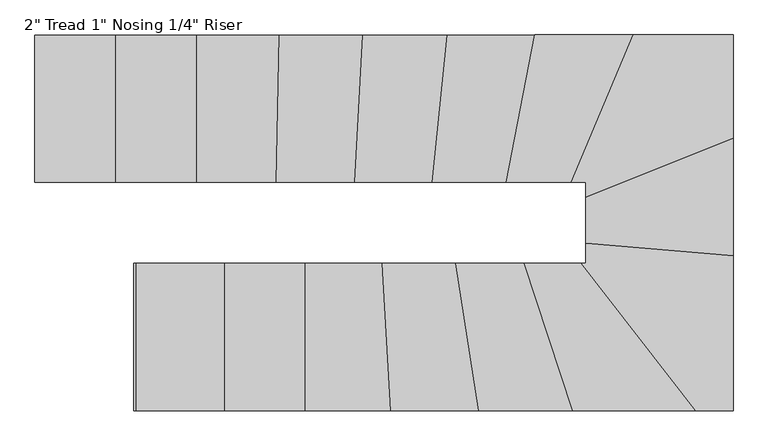
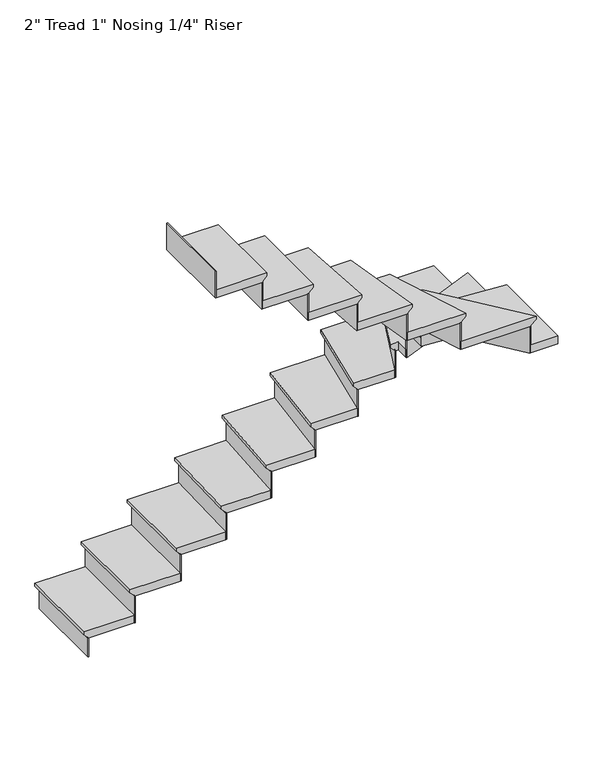
"""IFC4 building model written with IfcOpenShell, lengths in millimetres: stair flight geometry."""

from ifc_helpers import new_model, si_unit, origin, place, context, project, spatial, faceted_brep, source, transform, mapped, element, save


def stair_flight_0d7771ed(model_context):
    return source(origin(), model_context, "Body", "Brep", [
        faceted_brep([(838.4202681, 2693.877558, 9920.8166667), (838.4202681, 2693.877558, 9939.8666667), (838.4202681, 3202.4524989, 9939.8666667), (838.4202681, 3202.4524989, 9920.8166667), (863.8202681, 2693.877558, 9895.4166667), (863.8202681, 3202.4524989, 9895.4166667), (1143.2202681, 2693.877558, 9939.8666667), (1143.2202681, 3202.4524989, 9939.8666667), (863.8202681, 3202.4524989, 9889.0666667), (1143.2202681, 3202.4524989, 9889.0666667), (1143.2202681, 2693.877558, 9889.0666667), (863.8202681, 2693.877558, 9889.0666667)], [[[0, 1, 2, 3]], [[4, 0, 3, 5]], [[2, 1, 6, 7]], [[8, 9, 10, 11]], [[2, 7, 9, 8, 5, 3]], [[8, 11, 4, 5]], [[6, 1, 0, 4, 11, 10]], [[7, 6, 10, 9]]]),
        faceted_brep([(863.8202681, 2693.877558, 9889.0666667), (863.8202681, 2693.877558, 9770.5333333), (870.1702681, 2693.877558, 9770.5333333), (870.1702681, 2693.877558, 9889.0666667), (863.8202681, 3202.4524989, 9889.0666667), (870.1702681, 3202.4524989, 9889.0666667), (870.1702681, 3202.4524989, 9770.5333333), (863.8202681, 3202.4524989, 9770.5333333)], [[[0, 1, 2, 3]], [[4, 5, 6, 7]], [[1, 0, 4, 7]], [[2, 1, 7, 6]], [[3, 2, 6, 5]], [[0, 3, 5, 4]]]),
        faceted_brep([(1143.2202681, 2693.877558, 10058.4), (1143.2202681, 2693.877558, 9889.0666667), (1149.5702681, 2693.877558, 9889.0666667), (1149.5702681, 2693.877558, 10058.4), (1143.2202681, 3202.4524989, 10058.4), (1149.5702681, 3202.4524989, 10058.4), (1149.5702681, 3202.4524989, 9889.0666667), (1143.2202681, 3202.4524989, 9889.0666667)], [[[0, 1, 2, 3]], [[4, 5, 6, 7]], [[1, 0, 4, 7]], [[2, 1, 7, 6]], [[3, 2, 6, 5]], [[0, 3, 5, 4]]]),
        faceted_brep([(1117.8202681, 3202.4524989, 10109.2), (1117.8202681, 2693.877558, 10109.2), (1422.6202681, 2693.877558, 10109.2), (1422.6202681, 3202.4524989, 10109.2), (1143.2202681, 3202.4524989, 10058.4), (1422.6202681, 3202.4524989, 10058.4), (1422.6202681, 2693.877558, 10058.4), (1143.2202681, 2693.877558, 10058.4), (1143.2202681, 3202.4524989, 10064.75), (1117.8202681, 3202.4524989, 10090.15), (1143.2202681, 2693.877558, 10064.75), (1117.8202681, 2693.877558, 10090.15)], [[[0, 1, 2, 3]], [[4, 5, 6, 7]], [[0, 3, 5, 4, 8, 9]], [[4, 7, 10, 8]], [[2, 1, 11, 10, 7, 6]], [[3, 2, 6, 5]], [[11, 1, 0, 9]], [[10, 11, 9, 8]]]),
        faceted_brep([(1422.6202681, 2693.877558, 10227.7333333), (1422.6202681, 2693.877558, 10058.4), (1428.9702681, 2693.877558, 10058.4), (1428.9702681, 2693.877558, 10227.7333333), (1422.6202681, 3202.4524989, 10227.7333333), (1428.9702681, 3202.4524989, 10227.7333333), (1428.9702681, 3202.4524989, 10058.4), (1422.6202681, 3202.4524989, 10058.4)], [[[0, 1, 2, 3]], [[4, 5, 6, 7]], [[1, 0, 4, 7]], [[2, 1, 7, 6]], [[3, 2, 6, 5]], [[0, 3, 5, 4]]]),
        faceted_brep([(1397.2202681, 3202.4524989, 10278.5333333), (1397.2202681, 2693.877558, 10278.5333333), (1696.6553711, 2693.877558, 10278.5333333), (1707.3964935, 3202.4524989, 10278.5333333), (1422.6202681, 3202.4524989, 10227.7333333), (1707.3964935, 3202.4524989, 10227.7333333), (1696.6553711, 2693.877558, 10227.7333333), (1422.6202681, 2693.877558, 10227.7333333), (1422.6202681, 3202.4524989, 10234.0833333), (1397.2202681, 3202.4524989, 10259.4833333), (1422.6202681, 2693.877558, 10234.0833333), (1397.2202681, 2693.877558, 10259.4833333)], [[[0, 1, 2, 3]], [[4, 5, 6, 7]], [[0, 3, 5, 4, 8, 9]], [[4, 7, 10, 8]], [[2, 1, 11, 10, 7, 6]], [[3, 2, 6, 5]], [[11, 1, 0, 9]], [[10, 11, 9, 8]]]),
        faceted_brep([(1696.6553711, 2693.877558, 10397.0666667), (1696.6553711, 2693.877558, 10227.7333333), (1703.0067872, 2693.877558, 10227.7333333), (1703.0067872, 2693.877558, 10397.0666667), (1707.3964935, 3202.4524989, 10397.0666667), (1713.7479096, 3202.4524989, 10397.0666667), (1713.7479096, 3202.4524989, 10227.7333333), (1707.3964935, 3202.4524989, 10227.7333333)], [[[0, 1, 2, 3]], [[4, 5, 6, 7]], [[1, 0, 4, 7]], [[2, 1, 7, 6]], [[3, 2, 6, 5]], [[0, 3, 5, 4]]]),
        faceted_brep([(1681.9908293, 3202.4524989, 10447.8666667), (1671.2497068, 2693.877558, 10447.8666667), (1968.2389719, 2693.877558, 10447.8666667), (1994.6701229, 3202.4524989, 10447.8666667), (1707.3964935, 3202.4524989, 10397.0666667), (1994.6701229, 3202.4524989, 10397.0666667), (1968.2389719, 2693.877558, 10397.0666667), (1696.6553711, 2693.877558, 10397.0666667), (1707.3964935, 3202.4524989, 10403.4166667), (1681.9908293, 3202.4524989, 10428.8166667), (1696.6553711, 2693.877558, 10403.4166667), (1671.2497068, 2693.877558, 10428.8166667)], [[[0, 1, 2, 3]], [[4, 5, 6, 7]], [[0, 3, 5, 4, 8, 9]], [[4, 7, 10, 8]], [[2, 1, 11, 10, 7, 6]], [[3, 2, 6, 5]], [[11, 1, 0, 9]], [[10, 11, 9, 8]]]),
        faceted_brep([(1968.2389719, 2693.877558, 10566.4), (1968.2389719, 2693.877558, 10397.0666667), (1974.5975418, 2693.877558, 10397.0666667), (1974.5975418, 2693.877558, 10566.4), (1994.6701229, 3202.4524989, 10566.4), (2001.0286928, 3202.4524989, 10566.4), (2001.0286928, 3202.4524989, 10397.0666667), (1994.6701229, 3202.4524989, 10397.0666667)], [[[0, 1, 2, 3]], [[4, 5, 6, 7]], [[1, 0, 4, 7]], [[2, 1, 7, 6]], [[3, 2, 6, 5]], [[0, 3, 5, 4]]]),
        faceted_brep([(1969.2358436, 3202.4524989, 10617.2), (1942.8046925, 2693.877558, 10617.2), (2235.1931673, 2693.877558, 10617.2), (2286.7073051, 3202.4524989, 10617.2), (1994.6701229, 3202.4524989, 10566.4), (2286.7073051, 3202.4524989, 10566.4), (2235.1931673, 2693.877558, 10566.4), (1968.2389719, 2693.877558, 10566.4), (1994.6701229, 3202.4524989, 10572.75), (1969.2358436, 3202.4524989, 10598.15), (1968.2389719, 2693.877558, 10572.75), (1942.8046925, 2693.877558, 10598.15)], [[[0, 1, 2, 3]], [[4, 5, 6, 7]], [[0, 3, 5, 4, 8, 9]], [[4, 7, 10, 8]], [[2, 1, 11, 10, 7, 6]], [[3, 2, 6, 5]], [[11, 1, 0, 9]], [[10, 11, 9, 8]]]),
        faceted_brep([(2235.1931673, 2693.877558, 10735.7333333), (2235.1931673, 2693.877558, 10566.4), (2241.5756594, 2693.877558, 10566.4), (2241.5756594, 2693.877558, 10735.7333333), (2286.7073051, 3202.4524989, 10735.7333333), (2293.0897971, 3202.4524989, 10735.7333333), (2293.0897971, 3202.4524989, 10566.4), (2286.7073051, 3202.4524989, 10566.4)], [[[0, 1, 2, 3]], [[4, 5, 6, 7]], [[1, 0, 4, 7]], [[2, 1, 7, 6]], [[3, 2, 6, 5]], [[0, 3, 5, 4]]]),
        faceted_brep([(2261.1773369, 3202.4524989, 10786.5333333), (2209.6631992, 2693.877558, 10786.5333333), (2491.6737127, 2693.877558, 10786.5333333), (2589.7018996, 3202.4524989, 10786.5333333), (2286.7073051, 3202.4524989, 10735.7333333), (2589.7018996, 3202.4524989, 10735.7333333), (2491.6737127, 2693.877558, 10735.7333333), (2235.1931673, 2693.877558, 10735.7333333), (2286.7073051, 3202.4524989, 10742.0833333), (2261.1773369, 3202.4524989, 10767.4833333), (2235.1931673, 2693.877558, 10742.0833333), (2209.6631992, 2693.877558, 10767.4833333)], [[[0, 1, 2, 3]], [[4, 5, 6, 7]], [[0, 3, 5, 4, 8, 9]], [[4, 7, 10, 8]], [[2, 1, 11, 10, 7, 6]], [[3, 2, 6, 5]], [[11, 1, 0, 9]], [[10, 11, 9, 8]]]),
        faceted_brep([(2491.6737127, 2693.877558, 10905.0666667), (2491.6737127, 2693.877558, 10735.7333333), (2498.1405972, 2693.877558, 10735.7333333), (2498.1405972, 2693.877558, 10905.0666667), (2589.7018996, 3202.4524989, 10905.0666667), (2596.1687841, 3202.4524989, 10905.0666667), (2596.1687841, 3202.4524989, 10735.7333333), (2589.7018996, 3202.4524989, 10735.7333333)], [[[0, 1, 2, 3]], [[4, 5, 6, 7]], [[1, 0, 4, 7]], [[2, 1, 7, 6]], [[3, 2, 6, 5]], [[0, 3, 5, 4]]]),
        faceted_brep([(2563.8343615, 3202.4524989, 10955.8666667), (2465.8061746, 2693.877558, 10955.8666667), (2717.082711, 2693.877558, 10955.8666667), (2931.3822032, 3202.4524989, 10955.8666667), (2589.7018996, 3202.4524989, 10905.0666667), (2931.3822032, 3202.4524989, 10905.0666667), (2717.082711, 2693.877558, 10905.0666667), (2491.6737127, 2693.877558, 10905.0666667), (2589.7018996, 3202.4524989, 10911.4166667), (2563.8343615, 3202.4524989, 10936.8166667), (2491.6737127, 2693.877558, 10911.4166667), (2465.8061746, 2693.877558, 10936.8166667)], [[[0, 1, 2, 3]], [[4, 5, 6, 7]], [[0, 3, 5, 4, 8, 9]], [[4, 7, 10, 8]], [[2, 1, 11, 10, 7, 6]], [[3, 2, 6, 5]], [[11, 1, 0, 9]], [[10, 11, 9, 8]]]),
        faceted_brep([(2717.082711, 2693.877558, 11074.4), (2717.082711, 2693.877558, 10905.0666667), (2723.973426, 2693.877558, 10905.0666667), (2723.973426, 2693.877558, 11074.4), (2931.3822032, 3202.4524989, 11074.4), (2938.2729181, 3202.4524989, 11074.4), (2938.2729181, 3202.4524989, 10905.0666667), (2931.3822032, 3202.4524989, 10905.0666667)], [[[0, 1, 2, 3]], [[4, 5, 6, 7]], [[1, 0, 4, 7]], [[2, 1, 7, 6]], [[3, 2, 6, 5]], [[0, 3, 5, 4]]]),
        faceted_brep([(3247.982332, 2818.4435318, 11125.2), (3247.982332, 3202.4524989, 11125.2), (2903.8193433, 3202.4524989, 11125.2), (2689.5198512, 2693.877558, 11125.2), (2739.4073911, 2693.877558, 11125.2), (2739.4073911, 2614.5975609, 11125.2), (3247.982332, 3202.4524989, 11074.4), (3247.982332, 2818.4435318, 11074.4), (2739.4073911, 2614.5975609, 11074.4), (2739.4073911, 2693.877558, 11074.4), (2717.082711, 2693.877558, 11074.4), (2931.3822032, 3202.4524989, 11074.4), (2717.082711, 2693.877558, 11080.75), (2931.3822032, 3202.4524989, 11080.75), (2689.5198512, 2693.877558, 11106.15), (2903.8193433, 3202.4524989, 11106.15)], [[[0, 1, 2, 3, 4, 5]], [[6, 7, 8, 9, 10, 11]], [[1, 0, 7, 6]], [[11, 10, 12, 13]], [[5, 4, 9, 8]], [[0, 5, 8, 7]], [[14, 3, 2, 15]], [[12, 14, 15, 13]], [[4, 3, 14, 12, 10, 9]], [[2, 1, 6, 11, 13, 15]]]),
        faceted_brep([(2739.4073911, 2614.5975609, 11243.7333333), (2739.4073911, 2614.5975609, 11074.4), (2739.4073911, 2607.7564709, 11074.4), (2739.4073911, 2607.7564709, 11243.7333333), (3247.982332, 2818.4435318, 11243.7333333), (3247.982332, 2811.6024418, 11243.7333333), (3247.982332, 2811.6024418, 11074.4), (3247.982332, 2818.4435318, 11074.4)], [[[0, 1, 2, 3]], [[4, 5, 6, 7]], [[1, 0, 4, 7]], [[2, 1, 7, 6]], [[3, 2, 6, 5]], [[0, 3, 5, 4]]]),
        faceted_brep([(3247.982332, 2845.807892, 11294.5333333), (2739.4073911, 2641.9619211, 11294.5333333), (2739.4073911, 2458.7583414, 11294.5333333), (3247.982332, 2415.6151582, 11294.5333333), (3247.982332, 2818.4435318, 11243.7333333), (3247.982332, 2415.6151582, 11243.7333333), (2739.4073911, 2458.7583414, 11243.7333333), (2739.4073911, 2614.5975609, 11243.7333333), (3247.982332, 2818.4435318, 11250.0833333), (3247.982332, 2845.807892, 11275.4833333), (2739.4073911, 2614.5975609, 11250.0833333), (2739.4073911, 2641.9619211, 11275.4833333)], [[[0, 1, 2, 3]], [[4, 5, 6, 7]], [[0, 3, 5, 4, 8, 9]], [[4, 7, 10, 8]], [[2, 1, 11, 10, 7, 6]], [[3, 2, 6, 5]], [[11, 1, 0, 9]], [[10, 11, 9, 8]]]),
        faceted_brep([(2739.4073911, 2458.7583414, 11413.0666667), (2739.4073911, 2458.7583414, 11243.7333333), (2739.4073911, 2452.3855338, 11243.7333333), (2739.4073911, 2452.3855338, 11413.0666667), (3247.982332, 2415.6151582, 11413.0666667), (3247.982332, 2409.2423506, 11413.0666667), (3247.982332, 2409.2423506, 11243.7333333), (3247.982332, 2415.6151582, 11243.7333333)], [[[0, 1, 2, 3]], [[4, 5, 6, 7]], [[1, 0, 4, 7]], [[2, 1, 7, 6]], [[3, 2, 6, 5]], [[0, 3, 5, 4]]]),
        faceted_brep([(3085.5772675, 1905.9026171, 11463.8666667), (3247.982332, 1905.9026171, 11463.8666667), (3247.982332, 2441.1063885, 11463.8666667), (2739.4073911, 2484.2495716, 11463.8666667), (2739.4073911, 2414.477558, 11463.8666667), (2689.4386829, 2414.477558, 11463.8666667), (3247.982332, 1905.9026171, 11413.0666667), (3085.5772675, 1905.9026171, 11413.0666667), (2689.4386829, 2414.477558, 11413.0666667), (2739.4073911, 2414.477558, 11413.0666667), (2739.4073911, 2458.7583414, 11413.0666667), (3247.982332, 2415.6151582, 11413.0666667), (2739.4073911, 2458.7583414, 11419.4166667), (3247.982332, 2415.6151582, 11419.4166667), (2739.4073911, 2484.2495716, 11444.8166667), (3247.982332, 2441.1063885, 11444.8166667)], [[[0, 1, 2, 3, 4, 5]], [[6, 7, 8, 9, 10, 11]], [[1, 0, 7, 6]], [[11, 10, 12, 13]], [[4, 3, 14, 12, 10, 9]], [[5, 4, 9, 8]], [[0, 5, 8, 7]], [[14, 3, 2, 15]], [[12, 14, 15, 13]], [[2, 1, 6, 11, 13, 15]]]),
        faceted_brep([(2689.4386829, 2414.477558, 11582.4), (2689.4386829, 2414.477558, 11413.0666667), (2681.3896615, 2414.477558, 11413.0666667), (2681.3896615, 2414.477558, 11582.4), (3085.5772675, 1905.9026171, 11582.4), (3077.5282461, 1905.9026171, 11582.4), (3077.5282461, 1905.9026171, 11413.0666667), (3085.5772675, 1905.9026171, 11413.0666667)], [[[0, 1, 2, 3]], [[4, 5, 6, 7]], [[1, 0, 4, 7]], [[2, 1, 7, 6]], [[3, 2, 6, 5]], [[0, 3, 5, 4]]]),
        faceted_brep([(3117.7733531, 1905.9026171, 11633.2), (2721.6347685, 2414.477558, 11633.2), (2498.169104, 2414.477558, 11633.2), (2665.6971357, 1905.9026171, 11633.2), (3085.5772675, 1905.9026171, 11582.4), (2665.6971357, 1905.9026171, 11582.4), (2498.169104, 2414.477558, 11582.4), (2689.4386829, 2414.477558, 11582.4), (3085.5772675, 1905.9026171, 11588.75), (3117.7733531, 1905.9026171, 11614.15), (2689.4386829, 2414.477558, 11588.75), (2721.6347685, 2414.477558, 11614.15)], [[[0, 1, 2, 3]], [[4, 5, 6, 7]], [[0, 3, 5, 4, 8, 9]], [[4, 7, 10, 8]], [[2, 1, 11, 10, 7, 6]], [[3, 2, 6, 5]], [[11, 1, 0, 9]], [[10, 11, 9, 8]]]),
        faceted_brep([(2498.169104, 2414.477558, 11751.7333333), (2498.169104, 2414.477558, 11582.4), (2491.4834592, 2414.477558, 11582.4), (2491.4834592, 2414.477558, 11751.7333333), (2665.6971357, 1905.9026171, 11751.7333333), (2659.0114908, 1905.9026171, 11751.7333333), (2659.0114908, 1905.9026171, 11582.4), (2665.6971357, 1905.9026171, 11582.4)], [[[0, 1, 2, 3]], [[4, 5, 6, 7]], [[1, 0, 4, 7]], [[2, 1, 7, 6]], [[3, 2, 6, 5]], [[0, 3, 5, 4]]]),
        faceted_brep([(2692.4397151, 1905.9026171, 11802.5333333), (2524.9116834, 2414.477558, 11802.5333333), (2264.2527614, 2414.477558, 11802.5333333), (2342.8948816, 1905.9026171, 11802.5333333), (2665.6971357, 1905.9026171, 11751.7333333), (2342.8948816, 1905.9026171, 11751.7333333), (2264.2527614, 2414.477558, 11751.7333333), (2498.169104, 2414.477558, 11751.7333333), (2665.6971357, 1905.9026171, 11758.0833333), (2692.4397151, 1905.9026171, 11783.4833333), (2498.169104, 2414.477558, 11758.0833333), (2524.9116834, 2414.477558, 11783.4833333)], [[[0, 1, 2, 3]], [[4, 5, 6, 7]], [[0, 3, 5, 4, 8, 9]], [[4, 7, 10, 8]], [[2, 1, 11, 10, 7, 6]], [[3, 2, 6, 5]], [[11, 1, 0, 9]], [[10, 11, 9, 8]]]),
        faceted_brep([(2264.2527614, 2414.477558, 11921.0666667), (2264.2527614, 2414.477558, 11751.7333333), (2257.827292, 2414.477558, 11751.7333333), (2257.827292, 2414.477558, 11921.0666667), (2342.8948816, 1905.9026171, 11921.0666667), (2336.4694122, 1905.9026171, 11921.0666667), (2336.4694122, 1905.9026171, 11751.7333333), (2342.8948816, 1905.9026171, 11751.7333333)], [[[0, 1, 2, 3]], [[4, 5, 6, 7]], [[1, 0, 4, 7]], [[2, 1, 7, 6]], [[3, 2, 6, 5]], [[0, 3, 5, 4]]]),
        faceted_brep([(2368.5967594, 1905.9026171, 11971.8666667), (2289.9546392, 2414.477558, 11971.8666667), (2009.2587296, 2414.477558, 11971.8666667), (2039.6023306, 1905.9026171, 11971.8666667), (2342.8948816, 1905.9026171, 11921.0666667), (2039.6023306, 1905.9026171, 11921.0666667), (2009.2587296, 2414.477558, 11921.0666667), (2264.2527614, 2414.477558, 11921.0666667), (2342.8948816, 1905.9026171, 11927.4166667), (2368.5967594, 1905.9026171, 11952.8166667), (2264.2527614, 2414.477558, 11927.4166667), (2289.9546392, 2414.477558, 11952.8166667)], [[[0, 1, 2, 3]], [[4, 5, 6, 7]], [[0, 3, 5, 4, 8, 9]], [[4, 7, 10, 8]], [[2, 1, 11, 10, 7, 6]], [[3, 2, 6, 5]], [[11, 1, 0, 9]], [[10, 11, 9, 8]]]),
        faceted_brep([(2009.2587296, 2414.477558, 12090.4), (2009.2587296, 2414.477558, 11921.0666667), (2002.8974373, 2414.477558, 11921.0666667), (2002.8974373, 2414.477558, 12090.4), (2039.6023306, 1905.9026171, 12090.4), (2033.2410383, 1905.9026171, 12090.4), (2033.2410383, 1905.9026171, 11921.0666667), (2039.6023306, 1905.9026171, 11921.0666667)], [[[0, 1, 2, 3]], [[4, 5, 6, 7]], [[1, 0, 4, 7]], [[2, 1, 7, 6]], [[3, 2, 6, 5]], [[0, 3, 5, 4]]]),
        faceted_brep([(2065.0474997, 1905.9026171, 12141.2), (2034.7038988, 2414.477558, 12141.2), (1745.0756993, 2414.477558, 12141.2), (1745.0756993, 1905.9026171, 12141.2), (2039.6023306, 1905.9026171, 12090.4), (1745.0756993, 1905.9026171, 12090.4), (1745.0756993, 2414.477558, 12090.4), (2009.2587296, 2414.477558, 12090.4), (2039.6023306, 1905.9026171, 12096.75), (2065.0474997, 1905.9026171, 12122.15), (2009.2587296, 2414.477558, 12096.75), (2034.7038988, 2414.477558, 12122.15)], [[[0, 1, 2, 3]], [[4, 5, 6, 7]], [[0, 3, 5, 4, 8, 9]], [[4, 7, 10, 8]], [[2, 1, 11, 10, 7, 6]], [[3, 2, 6, 5]], [[11, 1, 0, 9]], [[10, 11, 9, 8]]]),
        faceted_brep([(1745.0756993, 2414.477558, 12259.7333333), (1745.0756993, 2414.477558, 12090.4), (1738.7256993, 2414.477558, 12090.4), (1738.7256993, 2414.477558, 12259.7333333), (1745.0756993, 1905.9026171, 12259.7333333), (1738.7256993, 1905.9026171, 12259.7333333), (1738.7256993, 1905.9026171, 12090.4), (1745.0756993, 1905.9026171, 12090.4)], [[[0, 1, 2, 3]], [[4, 5, 6, 7]], [[1, 0, 4, 7]], [[2, 1, 7, 6]], [[3, 2, 6, 5]], [[0, 3, 5, 4]]]),
        faceted_brep([(1770.4756993, 1905.9026171, 12310.5333333), (1770.4756993, 2414.477558, 12310.5333333), (1465.6756993, 2414.477558, 12310.5333333), (1465.6756993, 1905.9026171, 12310.5333333), (1745.0756993, 1905.9026171, 12259.7333333), (1465.6756993, 1905.9026171, 12259.7333333), (1465.6756993, 2414.477558, 12259.7333333), (1745.0756993, 2414.477558, 12259.7333333), (1745.0756993, 1905.9026171, 12266.0833333), (1770.4756993, 1905.9026171, 12291.4833333), (1745.0756993, 2414.477558, 12266.0833333), (1770.4756993, 2414.477558, 12291.4833333)], [[[0, 1, 2, 3]], [[4, 5, 6, 7]], [[0, 3, 5, 4, 8, 9]], [[4, 7, 10, 8]], [[2, 1, 11, 10, 7, 6]], [[3, 2, 6, 5]], [[11, 1, 0, 9]], [[10, 11, 9, 8]]]),
        faceted_brep([(1465.6756993, 2414.477558, 12429.0666667), (1465.6756993, 2414.477558, 12259.7333333), (1459.3256993, 2414.477558, 12259.7333333), (1459.3256993, 2414.477558, 12429.0666667), (1465.6756993, 1905.9026171, 12429.0666667), (1459.3256993, 1905.9026171, 12429.0666667), (1459.3256993, 1905.9026171, 12259.7333333), (1465.6756993, 1905.9026171, 12259.7333333)], [[[0, 1, 2, 3]], [[4, 5, 6, 7]], [[1, 0, 4, 7]], [[2, 1, 7, 6]], [[3, 2, 6, 5]], [[0, 3, 5, 4]]]),
        faceted_brep([(1186.2756993, 2414.477558, 12598.4), (1186.2756993, 2414.477558, 12429.0666667), (1179.9256993, 2414.477558, 12429.0666667), (1179.9256993, 2414.477558, 12598.4), (1186.2756993, 1905.9026171, 12598.4), (1179.9256993, 1905.9026171, 12598.4), (1179.9256993, 1905.9026171, 12429.0666667), (1186.2756993, 1905.9026171, 12429.0666667)], [[[0, 1, 2, 3]], [[4, 5, 6, 7]], [[1, 0, 4, 7]], [[2, 1, 7, 6]], [[3, 2, 6, 5]], [[0, 3, 5, 4]]]),
        faceted_brep([(1491.0756993, 1905.9026171, 12479.8666667), (1491.0756993, 2414.477558, 12479.8666667), (1186.2756993, 2414.477558, 12479.8666667), (1186.2756993, 1905.9026171, 12479.8666667), (1465.6756993, 1905.9026171, 12429.0666667), (1186.2756993, 1905.9026171, 12429.0666667), (1186.2756993, 2414.477558, 12429.0666667), (1465.6756993, 2414.477558, 12429.0666667), (1465.6756993, 1905.9026171, 12435.4166667), (1491.0756993, 1905.9026171, 12460.8166667), (1465.6756993, 2414.477558, 12435.4166667), (1491.0756993, 2414.477558, 12460.8166667)], [[[0, 1, 2, 3]], [[4, 5, 6, 7]], [[0, 3, 5, 4, 8, 9]], [[4, 7, 10, 8]], [[2, 1, 11, 10, 7, 6]], [[3, 2, 6, 5]], [[11, 1, 0, 9]], [[10, 11, 9, 8]]]),
    ])


if __name__ == "__main__":
    model = new_model("IFC4")
    model_context = context("Model", 3, world=origin())
    ifc_project = project(units=[si_unit("LENGTHUNIT", "METRE", prefix="MILLI")], contexts=[model_context])
    site = spatial("IfcSite", under=ifc_project)
    building = spatial("IfcBuilding", under=site)
    placement = place(None, origin())
    stair_flight_shape = stair_flight_0d7771ed(model_context)
    element("IfcStairFlight", 1, ObjectType="2\" Tread 1\" Nosing 1/4\" Riser", at=placement, inside=building, context=model_context, shape_type="MappedRepresentation", body=[
        mapped(stair_flight_shape, transform((0.0, 0.0, 0.0), x_axis=(1.0, 0.0, 0.0), y_axis=(0.0, 1.0, 0.0), z_axis=(0.0, 0.0, 1.0))),
    ])
    save(model, "model.ifc")
